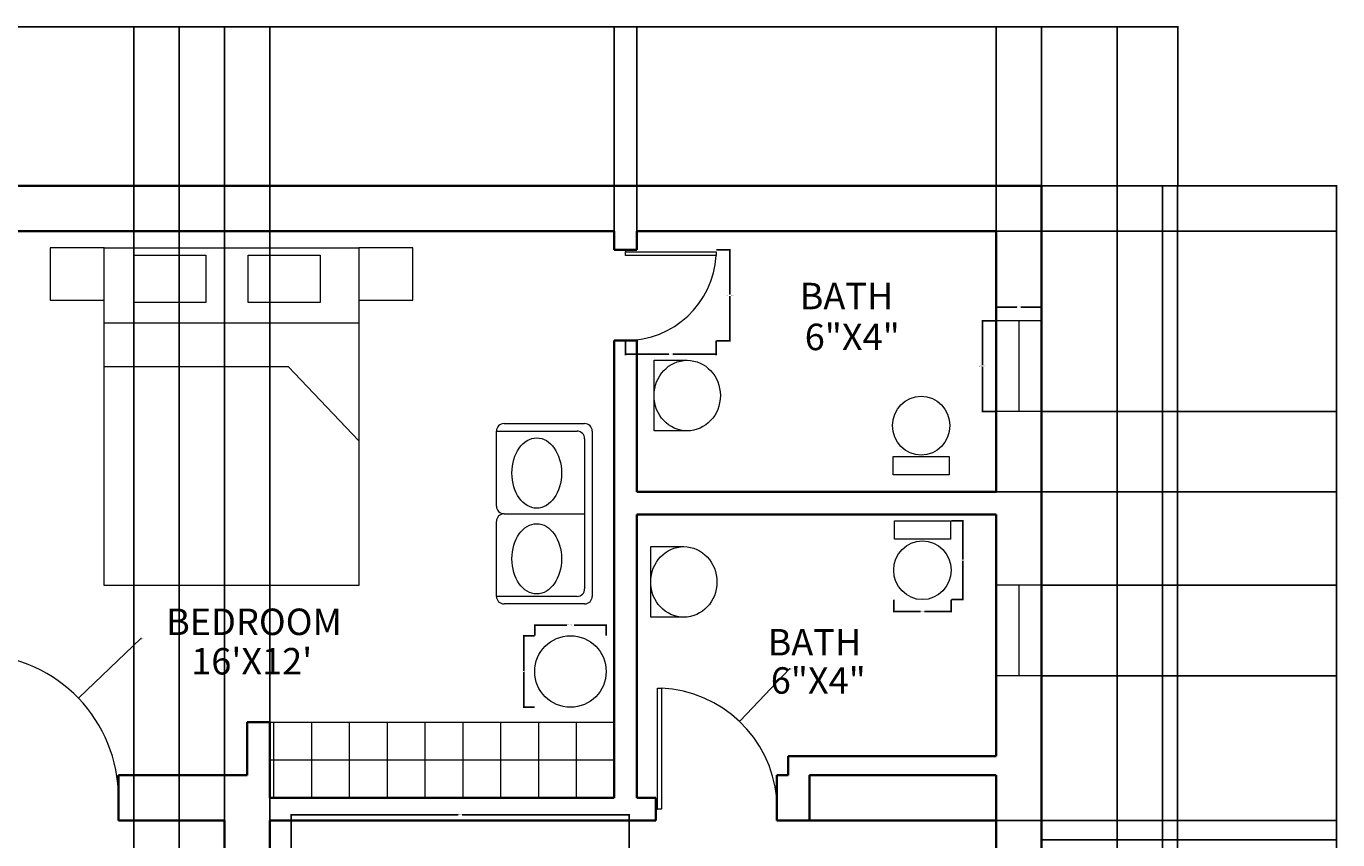
# Model space of a CAD drawing. Units: inches. Extents: x 2863 to 3499, y 1212 to 2136.
# Tile 7 of 7: x 3153 to 3499, y 1921 to 2136. Entities that reach past the tile are written whole.
import ezdxf

# ---------------------------------------------------------------- set-up
doc = ezdxf.new("R2010")
doc.units = ezdxf.units.IN
for name, color, linetype, lineweight in [('A-ANNO-DIMS', 2, 'Continuous', 18), ('A-AREA-IDEN', 7, 'Continuous', 18), ('A-DOOR', 221, 'Continuous', 18), ('A-FLOR-CASE', 254, 'Continuous', 18), ('A-FLOR-FIXT', 254, 'Continuous', 18), ('A-FURN', 131, 'Continuous', 18), ('A-GLAZ', 191, 'Continuous', 18), ('A-WALL', 51, 'Continuous', 35), ('C-PROP', 51, 'Continuous', 25)]:
    doc.layers.add(name, color=color, linetype=linetype, lineweight=lineweight)
doc.styles.get("Standard").update_dxf_attribs({"font": 'arial.ttf'})
doc.dimstyles.get("Standard").update_dxf_attribs({"dimtxt": 0.18, "dimasz": 0.18, "dimexe": 0.18, "dimexo": 0.0625, "dimgap": 0.09, "dimtad": 0, "dimtih": 1, "dimtoh": 1, "dimdec": 4, "dimzin": 0, "dimdsep": 46, "dimtxsty": 'Standard', "dimcen": 0.09, "dimadec": 0, "dimazin": 0, "dimtfac": 1, "dimtdec": 4, "dimtofl": 0, "dimtmove": 0, "dimatfit": 3, "dimfxl": 1, "dimtolj": 1, "dimtzin": 0, "dimarcsym": 0})

# ---------------------------------------------------------------- blocks, each defined once
blk = doc.blocks.new('SOFA-TWO-SEAT')
for p, q in [((0, 45.71), (21.32, 45.71)), ((0, 25.85), (0, 45.71)), ((2, 47.71), (23.32, 47.71)), ((25.32, 45.71), (25.32, 2)), ((23.32, 43.71), (23.32, 4)), ((0, 2), (0, 21.85)), ((2, 23.85), (23.32, 23.85)), ((2, 23.85), (2, 23.85)), ((21.32, 2), (0, 2)), ((23.32, 0), (2, 0))]:
    blk.add_line(p, q)
for centre, start, end in [((2, 45.71), 90, 180), ((21.32, 43.71), 0, 90), ((23.32, 45.71), 0, 90), ((2, 25.85), 180, 270), ((2, 21.85), 90, 180), ((21.32, 4), 270, 0), ((2, 2), 180, 270), ((23.32, 2), 270, 0)]:
    blk.add_arc(centre, 2, start, end)
for centre in [(10.66, 34.63), (10.66, 11.93)]:
    blk.add_ellipse(centre, major_axis=(0, 9.3), ratio=0.704902)
blk = doc.blocks.new('BED-DOUBLE-WITH-NIGHTSTANDS')
for p, q in [((19.89, 14.28), (19.89, 81.52)), ((31.47, 62.91), (51.09, 81.52)), ((31.47, 14.28), (31.47, 62.91))]:
    blk.add_line(p, q)
for points in [[(0, 81.52), (13.89, 81.52), (13.89, 95.8), (0, 95.8)], [(0, 81.52), (89.37, 81.52), (89.37, 14.28), (0, 14.28)], [(2, 71.31), (14.52, 71.31), (14.52, 52.28), (2, 52.28)], [(2, 41.11), (14.52, 41.11), (14.52, 22.08), (2, 22.08)], [(0, 0), (13.89, 0), (13.89, 14.28), (0, 14.28)]]:
    blk.add_lwpolyline(points, close=True)
blk = doc.blocks.new('WC-CLOSE-COUPLED')
blk.add_lwpolyline([(0.19, 20.82), (15, 20.82), (15, 15.96), (0.19, 15.96)], close=True)
blk.add_ellipse((7.6, 7.79), major_axis=(0, 7.78), ratio=0.975839)
blk = doc.blocks.new('TABLE-SIDE-ROUND')
blk.add_circle((9.45, 9.45), 9.45)
blk = doc.blocks.new('BASIN-WALL')
for p, q in [((8.77, 18.68), (17.53, 18.68)), ((17.53, 18.68), (17.53, 0)), ((17.53, 0), (8.77, 0))]:
    blk.add_line(p, q)
blk.add_ellipse((8.77, 9.34), major_axis=(0, 9.34), ratio=0.938307)
blk = doc.blocks.new('DOOR-SWING-24IN')
for p, q in [((0, 0.5), (0, 1.5)), ((0, 1.5), (24, 1.5)), ((24, 0.5), (0, 0.5)), ((24, 1.5), (24, 0.5)), ((24, 0), (24, 0.5))]:
    blk.add_line(p, q)
blk.add_arc((23.95, 0), 24, 89.888, 176.4168)
blk = doc.blocks.new('WINDOW-24IN')
for p, q in [((12, 24), (0, 24)), ((6, 24), (6, 0)), ((12, 0), (0, 0))]:
    blk.add_line(p, q)
blk = doc.blocks.new('*D23')
at = {"layer": 'A-ANNO-DIMS', "color": 0, "lineweight": -2, "transparency": 16777216}
for p, q in [((3397.1, 2005.45), (3400.34, 2005.45)), ((3400.16, 2005.27), (3400.16, 1995.22)), ((3400.16, 1984.81), (3400.16, 1994.86)), ((3397.1, 1984.63), (3400.34, 1984.63))]:
    blk.add_line(p, q, dxfattribs=at)
at = {"layer": 'A-ANNO-DIMS', "color": 0, "transparency": 16777216}
for points in [[(3400.13, 2005.27), (3400.19, 2005.27), (3400.16, 2005.45)], [(3400.13, 1984.81), (3400.19, 1984.81), (3400.16, 1984.63)]]:
    blk.add_solid(points, dxfattribs=at)
at = {"layer": 'Defpoints', "color": 0, "transparency": 16777216}
for p in [(3397.04, 2005.45), (3400.16, 2005.45), (3397.04, 1984.63)]:
    blk.add_point(p, dxfattribs=at)
at = {"layer": 'A-ANNO-DIMS', "color": 0, "transparency": 16777216, "insert": (3400.16, 1995.04), "char_height": 0.18, "attachment_point": 5}
blk.add_mtext('\\A1;WC 21 TYP.', dxfattribs=at)
blk = doc.blocks.new('*D24')
at = {"layer": 'A-ANNO-DIMS', "color": 0, "lineweight": -2, "transparency": 16777216}
for p, q in [((3381.84, 1984.56), (3381.84, 1981.32)), ((3397.04, 1984.56), (3397.04, 1981.32)), ((3382.02, 1981.5), (3388.92, 1981.5)), ((3396.86, 1981.5), (3389.96, 1981.5))]:
    blk.add_line(p, q, dxfattribs=at)
at = {"layer": 'A-ANNO-DIMS', "color": 0, "transparency": 16777216}
for points in [[(3382.02, 1981.53), (3382.02, 1981.47), (3381.84, 1981.5)], [(3396.86, 1981.53), (3396.86, 1981.47), (3397.04, 1981.5)]]:
    blk.add_solid(points, dxfattribs=at)
at = {"layer": 'Defpoints', "color": 0, "transparency": 16777216}
for p in [(3381.84, 1984.63), (3397.04, 1984.63), (3397.04, 1981.5)]:
    blk.add_point(p, dxfattribs=at)
at = {"layer": 'A-ANNO-DIMS', "color": 0, "transparency": 16777216, "insert": (3389.44, 1981.5), "char_height": 0.18, "attachment_point": 5}
blk.add_mtext('\\A1;15 TYP.', dxfattribs=at)
blk = doc.blocks.new('*D25')
at = {"layer": 'A-ANNO-DIMS', "color": 0, "lineweight": -2, "transparency": 16777216}
for p, q in [((3286.93, 1975.12), (3286.93, 1978.07)), ((3287.11, 1977.89), (3295.41, 1977.89)), ((3305.65, 1977.89), (3297.34, 1977.89)), ((3305.83, 1975.12), (3305.83, 1978.07))]:
    blk.add_line(p, q, dxfattribs=at)
at = {"layer": 'A-ANNO-DIMS', "color": 0, "transparency": 16777216}
for points in [[(3287.11, 1977.92), (3287.11, 1977.86), (3286.93, 1977.89)], [(3305.65, 1977.92), (3305.65, 1977.86), (3305.83, 1977.89)]]:
    blk.add_solid(points, dxfattribs=at)
at = {"layer": 'Defpoints', "color": 0, "transparency": 16777216}
for p in [(3305.83, 1977.89), (3286.93, 1975.05), (3305.83, 1975.05)]:
    blk.add_point(p, dxfattribs=at)
at = {"layer": 'A-ANNO-DIMS', "color": 0, "transparency": 16777216, "insert": (3296.38, 1977.89), "char_height": 0.18, "attachment_point": 5}
blk.add_mtext('\\A1;TABLE 19 TYP.', dxfattribs=at)
blk = doc.blocks.new('*D26')
at = {"layer": 'A-ANNO-DIMS', "color": 0, "lineweight": -2, "transparency": 16777216}
for p, q in [((3286.87, 1975.05), (3283.91, 1975.05)), ((3284.09, 1974.87), (3284.09, 1965.79)), ((3284.09, 1956.34), (3284.09, 1965.42)), ((3286.87, 1956.16), (3283.91, 1956.16))]:
    blk.add_line(p, q, dxfattribs=at)
at = {"layer": 'A-ANNO-DIMS', "color": 0, "transparency": 16777216}
for points in [[(3284.06, 1974.87), (3284.12, 1974.87), (3284.09, 1975.05)], [(3284.06, 1956.34), (3284.12, 1956.34), (3284.09, 1956.16)]]:
    blk.add_solid(points, dxfattribs=at)
at = {"layer": 'Defpoints', "color": 0, "transparency": 16777216}
for p in [(3284.09, 1975.05), (3286.93, 1975.05), (3286.93, 1956.16)]:
    blk.add_point(p, dxfattribs=at)
at = {"layer": 'A-ANNO-DIMS', "color": 0, "transparency": 16777216, "insert": (3284.09, 1965.6), "char_height": 0.18, "attachment_point": 5}
blk.add_mtext('\\A1;19 TYP.', dxfattribs=at)
blk = doc.blocks.new('*D31')
at = {"layer": 'A-ANNO-DIMS', "color": 0, "lineweight": -2, "transparency": 16777216}
for p, q in [((3408.85, 2058.44), (3405.14, 2058.44)), ((3405.32, 2058.26), (3405.32, 2046.63)), ((3405.32, 2034.62), (3405.32, 2046.26)), ((3408.85, 2034.44), (3405.14, 2034.44))]:
    blk.add_line(p, q, dxfattribs=at)
at = {"layer": 'A-ANNO-DIMS', "color": 0, "transparency": 16777216}
for points in [[(3405.29, 2058.26), (3405.35, 2058.26), (3405.32, 2058.44)], [(3405.29, 2034.62), (3405.35, 2034.62), (3405.32, 2034.44)]]:
    blk.add_solid(points, dxfattribs=at)
at = {"layer": 'Defpoints', "color": 0, "transparency": 16777216}
for p in [(3405.32, 2058.44), (3408.92, 2058.44), (3408.92, 2034.44)]:
    blk.add_point(p, dxfattribs=at)
at = {"layer": 'A-ANNO-DIMS', "color": 0, "transparency": 16777216, "insert": (3405.32, 2046.44), "char_height": 0.18, "attachment_point": 5}
blk.add_mtext('\\A1;WINDOW 24 TYP.', dxfattribs=at)
blk = doc.blocks.new('*D32')
at = {"layer": 'A-ANNO-DIMS', "color": 0, "lineweight": -2, "transparency": 16777216}
for p, q in [((3408.92, 2058.51), (3408.92, 2062.22)), ((3409.1, 2062.04), (3414.4, 2062.04)), ((3420.74, 2062.04), (3415.44, 2062.04)), ((3420.92, 2058.51), (3420.92, 2062.22))]:
    blk.add_line(p, q, dxfattribs=at)
at = {"layer": 'A-ANNO-DIMS', "color": 0, "transparency": 16777216}
for points in [[(3409.1, 2062.07), (3409.1, 2062.01), (3408.92, 2062.04)], [(3420.74, 2062.07), (3420.74, 2062.01), (3420.92, 2062.04)]]:
    blk.add_solid(points, dxfattribs=at)
at = {"layer": 'Defpoints', "color": 0, "transparency": 16777216}
for p in [(3420.92, 2062.04), (3408.92, 2058.44), (3420.92, 2058.44)]:
    blk.add_point(p, dxfattribs=at)
at = {"layer": 'A-ANNO-DIMS', "color": 0, "transparency": 16777216, "insert": (3414.92, 2062.04), "char_height": 0.18, "attachment_point": 5}
blk.add_mtext('\\A1;12 TYP.', dxfattribs=at)
blk = doc.blocks.new('*D36')
at = {"layer": 'A-ANNO-DIMS', "color": 0, "lineweight": -2, "transparency": 16777216}
for p, q in [((3222.54, 1913.39), (3222.54, 1927.87)), ((3311.9, 1913.39), (3311.9, 1927.87)), ((3222.72, 1927.69), (3266.69, 1927.69)), ((3311.72, 1927.69), (3267.75, 1927.69))]:
    blk.add_line(p, q, dxfattribs=at)
at = {"layer": 'A-ANNO-DIMS', "color": 0, "transparency": 16777216}
for points in [[(3222.72, 1927.72), (3222.72, 1927.66), (3222.54, 1927.69)], [(3311.72, 1927.72), (3311.72, 1927.66), (3311.9, 1927.69)]]:
    blk.add_solid(points, dxfattribs=at)
at = {"layer": 'Defpoints', "color": 0, "transparency": 16777216}
for p in [(3311.9, 1927.69), (3222.54, 1913.32), (3311.9, 1913.32)]:
    blk.add_point(p, dxfattribs=at)
at = {"layer": 'A-ANNO-DIMS', "color": 0, "transparency": 16777216, "insert": (3267.22, 1927.69), "char_height": 0.18, "attachment_point": 5}
blk.add_mtext('\\A1;89 TYP.', dxfattribs=at)
blk = doc.blocks.new('*D43')
at = {"layer": 'A-ANNO-DIMS', "color": 0, "lineweight": -2, "transparency": 16777216}
for p, q in [((3334.98, 2077.17), (3338.7, 2077.17)), ((3338.52, 2076.99), (3338.52, 2065.34)), ((3338.52, 2053.32), (3338.52, 2064.97)), ((3334.98, 2053.14), (3338.7, 2053.14))]:
    blk.add_line(p, q, dxfattribs=at)
at = {"layer": 'A-ANNO-DIMS', "color": 0, "transparency": 16777216}
for points in [[(3338.49, 2076.99), (3338.55, 2076.99), (3338.52, 2077.17)], [(3338.49, 2053.32), (3338.55, 2053.32), (3338.52, 2053.14)]]:
    blk.add_solid(points, dxfattribs=at)
at = {"layer": 'Defpoints', "color": 0, "transparency": 16777216}
for p in [(3334.92, 2077.17), (3334.92, 2053.14), (3338.52, 2053.14)]:
    blk.add_point(p, dxfattribs=at)
at = {"layer": 'A-ANNO-DIMS', "color": 0, "transparency": 16777216, "insert": (3338.52, 2065.15), "char_height": 0.18, "attachment_point": 5}
blk.add_mtext('\\A1;BATH DOOR 24 TYP.', dxfattribs=at)
blk = doc.blocks.new('*D44')
at = {"layer": 'A-ANNO-DIMS', "color": 0, "lineweight": -2, "transparency": 16777216}
for p, q in [((3310.92, 2053.08), (3310.92, 2049.36)), ((3334.92, 2053.08), (3334.92, 2049.36)), ((3311.1, 2049.54), (3322.39, 2049.54)), ((3334.74, 2049.54), (3323.45, 2049.54))]:
    blk.add_line(p, q, dxfattribs=at)
at = {"layer": 'A-ANNO-DIMS', "color": 0, "transparency": 16777216}
for points in [[(3311.1, 2049.57), (3311.1, 2049.51), (3310.92, 2049.54)], [(3334.74, 2049.57), (3334.74, 2049.51), (3334.92, 2049.54)]]:
    blk.add_solid(points, dxfattribs=at)
at = {"layer": 'Defpoints', "color": 0, "transparency": 16777216}
for p in [(3310.92, 2053.14), (3334.92, 2053.14), (3310.92, 2049.54)]:
    blk.add_point(p, dxfattribs=at)
at = {"layer": 'A-ANNO-DIMS', "color": 0, "transparency": 16777216, "insert": (3322.92, 2049.54), "char_height": 0.18, "attachment_point": 5}
blk.add_mtext('\\A1;24 TYP.', dxfattribs=at)
blk = doc.blocks.new('*D52')
at = {"layer": 'A-ANNO-DIMS', "color": 0, "lineweight": -2, "transparency": 16777216}
for p, q in [((2940.92, 2094.23), (2940.92, 2136.37)), ((2941.1, 2136.19), (3180.62, 2136.19)), ((3420.74, 2136.19), (3181.21, 2136.19)), ((3420.92, 2094.23), (3420.92, 2136.37))]:
    blk.add_line(p, q, dxfattribs=at)
at = {"layer": 'A-ANNO-DIMS', "color": 0, "transparency": 16777216}
for points in [[(2941.1, 2136.22), (2941.1, 2136.16), (2940.92, 2136.19)], [(3420.74, 2136.22), (3420.74, 2136.16), (3420.92, 2136.19)]]:
    blk.add_solid(points, dxfattribs=at)
at = {"layer": 'Defpoints', "color": 0, "transparency": 16777216}
for p in [(3420.92, 2136.19), (2940.92, 2094.17), (3420.92, 2094.17)]:
    blk.add_point(p, dxfattribs=at)
at = {"layer": 'A-ANNO-DIMS', "color": 0, "transparency": 16777216, "insert": (3180.92, 2136.19), "char_height": 0.18, "attachment_point": 5}
blk.add_mtext('\\A1;480', dxfattribs=at)
blk = doc.blocks.new('*D53')
at = {"layer": 'A-ANNO-DIMS', "color": 0, "lineweight": -2, "transparency": 16777216}
for p, q in [((3420.92, 2094.23), (3420.92, 2136.37)), ((3421.1, 2136.19), (3438.7, 2136.19)), ((3456.74, 2136.19), (3439.14, 2136.19)), ((3456.92, 2094.23), (3456.92, 2136.37))]:
    blk.add_line(p, q, dxfattribs=at)
at = {"layer": 'A-ANNO-DIMS', "color": 0, "transparency": 16777216}
for points in [[(3421.1, 2136.22), (3421.1, 2136.16), (3420.92, 2136.19)], [(3456.74, 2136.22), (3456.74, 2136.16), (3456.92, 2136.19)]]:
    blk.add_solid(points, dxfattribs=at)
at = {"layer": 'Defpoints', "color": 0, "transparency": 16777216}
for p in [(3456.92, 2136.19), (3420.92, 2094.17), (3456.92, 2094.17)]:
    blk.add_point(p, dxfattribs=at)
at = {"layer": 'A-ANNO-DIMS', "color": 0, "transparency": 16777216, "insert": (3438.92, 2136.19), "char_height": 0.18, "attachment_point": 5}
blk.add_mtext('\\A1;36', dxfattribs=at)
blk = doc.blocks.new('*D55')
at = {"layer": 'A-ANNO-DIMS', "color": 0, "lineweight": -2, "transparency": 16777216}
for p, q in [((3115.92, 2082.23), (3115.92, 2136.37)), ((3116.1, 2136.19), (3211.64, 2136.19)), ((3307.74, 2136.19), (3212.2, 2136.19)), ((3307.92, 2082.23), (3307.92, 2136.37))]:
    blk.add_line(p, q, dxfattribs=at)
at = {"layer": 'A-ANNO-DIMS', "color": 0, "transparency": 16777216}
for points in [[(3116.1, 2136.22), (3116.1, 2136.16), (3115.92, 2136.19)], [(3307.74, 2136.22), (3307.74, 2136.16), (3307.92, 2136.19)]]:
    blk.add_solid(points, dxfattribs=at)
at = {"layer": 'Defpoints', "color": 0, "transparency": 16777216}
for p in [(3307.92, 2136.19), (3115.92, 2082.17), (3307.92, 2082.17)]:
    blk.add_point(p, dxfattribs=at)
at = {"layer": 'A-ANNO-DIMS', "color": 0, "transparency": 16777216, "insert": (3211.92, 2136.19), "char_height": 0.18, "attachment_point": 5}
blk.add_mtext('\\A1;192', dxfattribs=at)
blk = doc.blocks.new('*D56')
at = {"layer": 'A-ANNO-DIMS', "color": 0, "lineweight": -2, "transparency": 16777216}
for p, q in [((3313.92, 2082.23), (3313.92, 2136.37)), ((3314.1, 2136.19), (3361.2, 2136.19)), ((3408.74, 2136.19), (3361.64, 2136.19)), ((3408.92, 2082.23), (3408.92, 2136.37))]:
    blk.add_line(p, q, dxfattribs=at)
at = {"layer": 'A-ANNO-DIMS', "color": 0, "transparency": 16777216}
for points in [[(3314.1, 2136.22), (3314.1, 2136.16), (3313.92, 2136.19)], [(3408.74, 2136.22), (3408.74, 2136.16), (3408.92, 2136.19)]]:
    blk.add_solid(points, dxfattribs=at)
at = {"layer": 'Defpoints', "color": 0, "transparency": 16777216}
for p in [(3408.92, 2136.19), (3313.92, 2082.17), (3408.92, 2082.17)]:
    blk.add_point(p, dxfattribs=at)
at = {"layer": 'A-ANNO-DIMS', "color": 0, "transparency": 16777216, "insert": (3361.42, 2136.19), "char_height": 0.18, "attachment_point": 5}
blk.add_mtext('\\A1;95', dxfattribs=at)
blk = doc.blocks.new('*D57')
at = {"layer": 'A-ANNO-DIMS', "color": 0, "lineweight": -2, "transparency": 16777216}
for p, q in [((3456.98, 2094.17), (3499.12, 2094.17)), ((3498.94, 2093.99), (3498.94, 1734.35)), ((3498.94, 1374.35), (3498.94, 1733.98)), ((3452.98, 1374.17), (3499.12, 1374.17))]:
    blk.add_line(p, q, dxfattribs=at)
at = {"layer": 'A-ANNO-DIMS', "color": 0, "transparency": 16777216}
for points in [[(3498.91, 2093.99), (3498.97, 2093.99), (3498.94, 2094.17)], [(3498.91, 1374.35), (3498.97, 1374.35), (3498.94, 1374.17)]]:
    blk.add_solid(points, dxfattribs=at)
at = {"layer": 'Defpoints', "color": 0, "transparency": 16777216}
for p in [(3456.92, 2094.17), (3498.94, 2094.17), (3452.92, 1374.17)]:
    blk.add_point(p, dxfattribs=at)
at = {"layer": 'A-ANNO-DIMS', "color": 0, "transparency": 16777216, "insert": (3498.94, 1734.17), "char_height": 0.18, "attachment_point": 5}
blk.add_mtext('\\A1;720', dxfattribs=at)
blk = doc.blocks.new('*D61')
at = {"layer": 'A-ANNO-DIMS', "color": 0, "lineweight": -2, "transparency": 16777216}
for p, q in [((3408.98, 1926.17), (3499.12, 1926.17)), ((3498.94, 1925.99), (3498.94, 1836.35)), ((3498.94, 1746.35), (3498.94, 1835.98)), ((3408.98, 1746.17), (3499.12, 1746.17))]:
    blk.add_line(p, q, dxfattribs=at)
at = {"layer": 'A-ANNO-DIMS', "color": 0, "transparency": 16777216}
for points in [[(3498.91, 1925.99), (3498.97, 1925.99), (3498.94, 1926.17)], [(3498.91, 1746.35), (3498.97, 1746.35), (3498.94, 1746.17)]]:
    blk.add_solid(points, dxfattribs=at)
at = {"layer": 'Defpoints', "color": 0, "transparency": 16777216}
for p in [(3408.92, 1926.17), (3498.94, 1926.17), (3408.92, 1746.17)]:
    blk.add_point(p, dxfattribs=at)
at = {"layer": 'A-ANNO-DIMS', "color": 0, "transparency": 16777216, "insert": (3498.94, 1836.17), "char_height": 0.18, "attachment_point": 5}
blk.add_mtext('\\A1;180', dxfattribs=at)
blk = doc.blocks.new('*D62')
at = {"layer": 'A-ANNO-DIMS', "color": 0, "lineweight": -2, "transparency": 16777216}
for p, q in [((3408.98, 2013.17), (3499.12, 2013.17)), ((3498.94, 2012.99), (3498.94, 1969.85)), ((3498.94, 1926.35), (3498.94, 1969.48)), ((3408.98, 1926.17), (3499.12, 1926.17))]:
    blk.add_line(p, q, dxfattribs=at)
at = {"layer": 'A-ANNO-DIMS', "color": 0, "transparency": 16777216}
for points in [[(3498.91, 2012.99), (3498.97, 2012.99), (3498.94, 2013.17)], [(3498.91, 1926.35), (3498.97, 1926.35), (3498.94, 1926.17)]]:
    blk.add_solid(points, dxfattribs=at)
at = {"layer": 'Defpoints', "color": 0, "transparency": 16777216}
for p in [(3408.92, 2013.17), (3498.94, 2013.17), (3408.92, 1926.17)]:
    blk.add_point(p, dxfattribs=at)
at = {"layer": 'A-ANNO-DIMS', "color": 0, "transparency": 16777216, "insert": (3498.94, 1969.67), "char_height": 0.18, "attachment_point": 5}
blk.add_mtext('\\A1;87', dxfattribs=at)
blk = doc.blocks.new('*D63')
at = {"layer": 'A-ANNO-DIMS', "color": 0, "lineweight": -2, "transparency": 16777216}
for p, q in [((3408.98, 2082.17), (3499.12, 2082.17)), ((3498.94, 2081.99), (3498.94, 2047.85)), ((3498.94, 2013.35), (3498.94, 2047.48)), ((3408.98, 2013.17), (3499.12, 2013.17))]:
    blk.add_line(p, q, dxfattribs=at)
at = {"layer": 'A-ANNO-DIMS', "color": 0, "transparency": 16777216}
for points in [[(3498.91, 2081.99), (3498.97, 2081.99), (3498.94, 2082.17)], [(3498.91, 2013.35), (3498.97, 2013.35), (3498.94, 2013.17)]]:
    blk.add_solid(points, dxfattribs=at)
at = {"layer": 'Defpoints', "color": 0, "transparency": 16777216}
for p in [(3408.92, 2082.17), (3498.94, 2082.17), (3408.92, 2013.17)]:
    blk.add_point(p, dxfattribs=at)
at = {"layer": 'A-ANNO-DIMS', "color": 0, "transparency": 16777216, "insert": (3498.94, 2047.67), "char_height": 0.18, "attachment_point": 5}
blk.add_mtext('\\A1;69', dxfattribs=at)
blk = doc.blocks.new('*D72')
at = {"layer": 'A-ANNO-DIMS', "color": 0, "lineweight": -2, "transparency": 16777216}
for p, q in [((3133.92, 1549.23), (3133.92, 2136.37)), ((3134.1, 2136.19), (3169.22, 2136.19)), ((3204.74, 2136.19), (3169.62, 2136.19)), ((3204.92, 1561.23), (3204.92, 2136.37))]:
    blk.add_line(p, q, dxfattribs=at)
at = {"layer": 'A-ANNO-DIMS', "color": 0, "transparency": 16777216}
for points in [[(3134.1, 2136.22), (3134.1, 2136.16), (3133.92, 2136.19)], [(3204.74, 2136.22), (3204.74, 2136.16), (3204.92, 2136.19)]]:
    blk.add_solid(points, dxfattribs=at)
at = {"layer": 'Defpoints', "color": 0, "transparency": 16777216}
for p in [(3204.92, 2136.19), (3204.92, 1561.17), (3133.92, 1549.17)]:
    blk.add_point(p, dxfattribs=at)
at = {"layer": 'A-ANNO-DIMS', "color": 0, "transparency": 16777216, "insert": (3169.42, 2136.19), "char_height": 0.18, "attachment_point": 5}
blk.add_mtext('\\A1;71', dxfattribs=at)
blk = doc.blocks.new('*D99')
at = {"layer": 'A-ANNO-DIMS', "color": 0, "lineweight": -2, "transparency": 16777216}
for p, q in [((3420.98, 1964.48), (3499.12, 1964.48)), ((3498.94, 1964.3), (3498.94, 1942.96)), ((3498.94, 1921.26), (3498.94, 1942.6)), ((3420.98, 1921.08), (3499.12, 1921.08))]:
    blk.add_line(p, q, dxfattribs=at)
at = {"layer": 'A-ANNO-DIMS', "color": 0, "transparency": 16777216}
for points in [[(3498.91, 1964.3), (3498.97, 1964.3), (3498.94, 1964.48)], [(3498.91, 1921.26), (3498.97, 1921.26), (3498.94, 1921.08)]]:
    blk.add_solid(points, dxfattribs=at)
at = {"layer": 'Defpoints', "color": 0, "transparency": 16777216}
for p in [(3420.92, 1964.48), (3498.94, 1964.48), (3420.92, 1921.08)]:
    blk.add_point(p, dxfattribs=at)
at = {"layer": 'A-ANNO-DIMS', "color": 0, "transparency": 16777216, "insert": (3498.94, 1942.78), "char_height": 0.18, "attachment_point": 5}
blk.add_mtext('\\A1;43.4', dxfattribs=at)
blk = doc.blocks.new('*D100')
at = {"layer": 'A-ANNO-DIMS', "color": 0, "lineweight": -2, "transparency": 16777216}
for p, q in [((3420.98, 2034.44), (3499.12, 2034.44)), ((3498.94, 2034.26), (3498.94, 2011.64)), ((3498.94, 1988.66), (3498.94, 2011.28)), ((3420.98, 1988.48), (3499.12, 1988.48))]:
    blk.add_line(p, q, dxfattribs=at)
at = {"layer": 'A-ANNO-DIMS', "color": 0, "transparency": 16777216}
for points in [[(3498.91, 2034.26), (3498.97, 2034.26), (3498.94, 2034.44)], [(3498.91, 1988.66), (3498.97, 1988.66), (3498.94, 1988.48)]]:
    blk.add_solid(points, dxfattribs=at)
at = {"layer": 'Defpoints', "color": 0, "transparency": 16777216}
for p in [(3420.92, 2034.44), (3498.94, 2034.44), (3420.92, 1988.48)]:
    blk.add_point(p, dxfattribs=at)
at = {"layer": 'A-ANNO-DIMS', "color": 0, "transparency": 16777216, "insert": (3498.94, 2011.46), "char_height": 0.18, "attachment_point": 5}
blk.add_mtext('\\A1;45.97', dxfattribs=at)
blk = doc.blocks.new('*D107')
at = {"layer": 'A-ANNO-DIMS', "color": 0, "lineweight": -2, "transparency": 16777216}
for p, q in [((3216.92, 1270.23), (3216.92, 2136.37)), ((3217.1, 2136.19), (3328.63, 2136.19)), ((3440.74, 2136.19), (3329.21, 2136.19)), ((3440.92, 1270.23), (3440.92, 2136.37))]:
    blk.add_line(p, q, dxfattribs=at)
at = {"layer": 'A-ANNO-DIMS', "color": 0, "transparency": 16777216}
for points in [[(3217.1, 2136.22), (3217.1, 2136.16), (3216.92, 2136.19)], [(3440.74, 2136.22), (3440.74, 2136.16), (3440.92, 2136.19)]]:
    blk.add_solid(points, dxfattribs=at)
at = {"layer": 'Defpoints', "color": 0, "transparency": 16777216}
for p in [(3440.92, 2136.19), (3216.92, 1270.17), (3440.92, 1270.17)]:
    blk.add_point(p, dxfattribs=at)
at = {"layer": 'A-ANNO-DIMS', "color": 0, "transparency": 16777216, "insert": (3328.92, 2136.19), "char_height": 0.18, "attachment_point": 5}
blk.add_mtext('\\A1;224', dxfattribs=at)
blk = doc.blocks.new('*D110')
at = {"layer": 'A-ANNO-DIMS', "color": 0, "lineweight": -2, "transparency": 16777216}
for p, q in [((3180.92, 1374.23), (3180.92, 2136.37)), ((3181.1, 2136.19), (3186.71, 2136.19)), ((3192.74, 2136.19), (3187.13, 2136.19)), ((3192.92, 1374.23), (3192.92, 2136.37))]:
    blk.add_line(p, q, dxfattribs=at)
at = {"layer": 'A-ANNO-DIMS', "color": 0, "transparency": 16777216}
for points in [[(3181.1, 2136.22), (3181.1, 2136.16), (3180.92, 2136.19)], [(3192.74, 2136.22), (3192.74, 2136.16), (3192.92, 2136.19)]]:
    blk.add_solid(points, dxfattribs=at)
at = {"layer": 'Defpoints', "color": 0, "transparency": 16777216}
for p in [(3192.92, 2136.19), (3180.92, 1374.17), (3192.92, 1374.17)]:
    blk.add_point(p, dxfattribs=at)
at = {"layer": 'A-ANNO-DIMS', "color": 0, "transparency": 16777216, "insert": (3186.92, 2136.19), "char_height": 0.18, "attachment_point": 5}
blk.add_mtext('\\A1;12', dxfattribs=at)
blk = doc.blocks.new('*D114')
at = {"layer": 'A-ANNO-DIMS', "color": 0, "lineweight": -2, "transparency": 16777216}
for p, q in [((3182.77, 1974.31), (3166.45, 1958.64)), ((3182.95, 1974.31), (3182.77, 1974.31)), ((3138.83, 1932.19), (3139.01, 1932.19)), ((3138.92, 1932.1), (3138.92, 1932.28))]:
    blk.add_line(p, q, dxfattribs=at)
at = {"layer": 'A-ANNO-DIMS', "color": 0, "transparency": 16777216}
blk.add_solid([(3166.43, 1958.66), (3166.47, 1958.62), (3166.32, 1958.52)], dxfattribs=at)
at = {"layer": 'Defpoints', "color": 0, "transparency": 16777216}
for p in [(3166.32, 1958.52), (3138.92, 1932.19)]:
    blk.add_point(p, dxfattribs=at)
at = {"layer": 'A-ANNO-DIMS', "color": 0, "transparency": 16777216, "insert": (3183.45, 1974.31), "char_height": 0.18, "attachment_point": 5}
blk.add_mtext('\\A1;2X R38', dxfattribs=at)
blk = doc.blocks.new('*D116')
at = {"layer": 'A-ANNO-DIMS', "color": 0, "lineweight": -2, "transparency": 16777216}
for p, q in [((3354.33, 1966.3), (3341.23, 1952.52)), ((3354.51, 1966.3), (3354.33, 1966.3)), ((3318.96, 1929.19), (3319.14, 1929.19)), ((3319.05, 1929.1), (3319.05, 1929.28))]:
    blk.add_line(p, q, dxfattribs=at)
at = {"layer": 'A-ANNO-DIMS', "color": 0, "transparency": 16777216}
blk.add_solid([(3341.21, 1952.54), (3341.25, 1952.49), (3341.1, 1952.38)], dxfattribs=at)
at = {"layer": 'Defpoints', "color": 0, "transparency": 16777216}
for p in [(3341.1, 1952.38), (3319.05, 1929.19)]:
    blk.add_point(p, dxfattribs=at)
at = {"layer": 'A-ANNO-DIMS', "color": 0, "transparency": 16777216, "insert": (3354.82, 1966.3), "char_height": 0.18, "attachment_point": 5}
blk.add_mtext('\\A1;R32', dxfattribs=at)

msp = doc.modelspace()

# ---------------------------------------------------------------- linework, layer by layer
at = {"layer": 'A-DOOR'}
for p, q in [((3319.4168, 1929.1651), (3319.4168, 1961.1651)), ((3319.4168, 1961.1651), (3320.4168, 1961.1651)), ((3320.4168, 1961.1651), (3320.4168, 1929.1651)), ((3318.9168, 1929.1651), (3319.4168, 1929.1651)), ((3320.4168, 1929.1651), (3319.4168, 1929.1651))]:
    msp.add_line(p, q, dxfattribs=at)
for centre, radius, start, end in [((3138.9168, 1932.1947), 38, 359.955345, 87.737754), ((3319.055, 1929.1941), 32, 5.327247, 87.561004)]:
    msp.add_arc(centre, radius, start, end, dxfattribs=at)
at = {"layer": 'A-FLOR-CASE'}
for p, q in [((3216.9168, 1952.1651), (3307.9168, 1952.1651)), ((3217.9168, 1952.1651), (3217.9168, 1932.1651)), ((3227.9168, 1952.1651), (3227.9168, 1932.1651)), ((3237.9168, 1952.1651), (3237.9168, 1932.1651)), ((3247.9168, 1952.1651), (3247.9168, 1932.1651)), ((3257.9168, 1952.1651), (3257.9168, 1932.1651)), ((3267.9168, 1952.1651), (3267.9168, 1932.1651)), ((3277.9168, 1952.1651), (3277.9168, 1932.1651)), ((3287.9168, 1952.1651), (3287.9168, 1932.1651)), ((3297.9168, 1952.1651), (3297.9168, 1932.1651)), ((3307.9168, 1952.1651), (3307.9168, 1932.1651)), ((3307.9168, 1942.1651), (3216.9168, 1942.1651))]:
    msp.add_line(p, q, dxfattribs=at)
at = {"layer": 'A-WALL'}
for p, q in [((3115.9168, 2082.1651), (3307.9168, 2082.1651)), ((3307.9168, 2082.1651), (3307.9168, 2077.1651)), ((3307.9168, 2077.1651), (3307.9168, 2082.1651)), ((3313.9168, 2082.1651), (3408.9168, 2082.1651)), ((3313.9168, 2077.1651), (3313.9168, 2082.1651)), ((3408.9168, 2082.1651), (3408.9168, 2013.1651)), ((3307.9168, 2077.1651), (3313.9168, 2077.1651)), ((3307.9168, 1938.1651), (3307.9168, 2053.1651)), ((3307.9168, 2053.1651), (3313.9168, 2053.1651)), ((3313.9168, 2013.1651), (3313.9168, 2053.1651)), ((3313.9168, 2013.1651), (3408.9168, 2013.1651)), ((3313.9168, 1938.1651), (3313.9168, 2007.1651)), ((3313.9168, 2007.1651), (3408.9168, 2007.1651)), ((3408.9168, 2007.1651), (3408.9168, 1943.1651)), ((3210.9168, 1938.1651), (3210.9168, 1952.1651)), ((3210.9168, 1952.1651), (3216.9168, 1952.1651)), ((3216.9168, 1952.1651), (3216.9168, 1938.1651)), ((3353.9168, 1938.1651), (3353.9168, 1943.1651)), ((3353.9168, 1943.1651), (3408.9168, 1943.1651)), ((3176.9168, 1926.1651), (3176.9168, 1938.1651)), ((3176.9168, 1938.1651), (3210.9168, 1938.1651)), ((3216.9168, 1938.1651), (3216.9168, 1932.1651)), ((3307.9168, 1932.1651), (3307.9168, 1938.1651)), ((3313.9168, 1938.1651), (3313.9168, 1932.1651)), ((3350.9168, 1938.1651), (3350.9168, 1926.1651)), ((3350.9168, 1938.1651), (3353.9168, 1938.1651)), ((3350.9168, 1938.1651), (3353.9168, 1938.1651)), ((3359.5654, 1938.1651), (3359.5654, 1926.1651)), ((3359.5654, 1938.1651), (3408.9168, 1938.1651)), ((3408.9168, 1938.1651), (3408.9168, 1926.1651)), ((3216.9168, 1932.1651), (3307.9168, 1932.1651)), ((3313.9168, 1932.1651), (3318.9168, 1932.1651)), ((3318.9168, 1932.1651), (3318.9168, 1926.1651)), ((3176.9168, 1926.1651), (3204.9168, 1926.1651)), ((3204.9168, 1926.1651), (3204.9168, 1806.1651)), ((3216.9168, 1926.1651), (3216.9168, 1806.1651)), ((3216.9168, 1926.1651), (3318.9168, 1926.1651)), ((3350.9168, 1926.1651), (3408.9168, 1926.1651)), ((3408.9168, 1926.1651), (3408.9168, 1561.1651))]:
    msp.add_line(p, q, dxfattribs=at)
msp.add_lwpolyline([(2940.9168, 1453.1651), (2940.9168, 2094.1651), (3420.9168, 2094.1651), (3420.9168, 1374.1651), (3216.9168, 1374.1651)], dxfattribs=at)
at = {"layer": 'C-PROP'}
for p, q in [((2904.9168, 2094.1651), (3456.9168, 2094.1651)), ((3456.9168, 2094.1651), (3420.9168, 2094.1651)), ((3452.9168, 1258.1651), (3452.9168, 2094.1651)), ((3456.9168, 2094.1651), (3456.9168, 1254.1651))]:
    msp.add_line(p, q, dxfattribs=at)

# ---------------------------------------------------------------- block references
at = {"layer": 'A-DOOR', "rotation": 180}
msp.add_blockref('DOOR-SWING-24IN', (3334.9165, 2077.1652), dxfattribs=at)
at = {"layer": 'A-FLOR-FIXT', "rotation": 180}
for name, p in [('BASIN-WALL', (3336.0181, 2047.9592)), ('WC-CLOSE-COUPLED', (3396.7096, 2038.4642)), ('BASIN-WALL', (3335.1328, 1998.6473))]:
    msp.add_blockref(name, p, dxfattribs=at)
at = {"layer": 'A-FLOR-FIXT'}
msp.add_blockref('WC-CLOSE-COUPLED', (3381.8439, 1984.6259), dxfattribs=at)
at = {"layer": 'A-FURN', "rotation": 269.9999999999988}
msp.add_blockref('BED-DOUBLE-WITH-NIGHTSTANDS', (3158.8772, 2077.7591), dxfattribs=at)
at = {"layer": 'A-FURN'}
for name, p in [('SOFA-TWO-SEAT', (3276.822, 1983.498)), ('TABLE-SIDE-ROUND', (3286.929, 1956.156))]:
    msp.add_blockref(name, p, dxfattribs=at)
at = {"layer": 'A-GLAZ'}
for p in [(3408.917, 2034.4449), (3408.917, 1964.4771)]:
    msp.add_blockref('WINDOW-24IN', p, dxfattribs=at)

# ---------------------------------------------------------------- texts
at = {"layer": 'A-AREA-IDEN'}
for tag, p in [('BATH', (3356.9751, 2061.4647)), ('6"X4"', (3358.3244, 2050.6453)), ('BEDROOM', (3189.4913, 1975.2591)), ('BATH', (3348.5033, 1969.8481)), ("16'X12'", (3196.136, 1964.8264)), ('6"X4"', (3349.3464, 1959.7363))]:
    msp.add_attdef(tag, p, '', height=7, dxfattribs=at)

# ---------------------------------------------------------------- dimensions: what is measured, and where the dimension line sits
at = {"layer": 'A-ANNO-DIMS'}
for base, p1, p2, picture, middle in [((3420.9168, 2136.1851), (2940.9168, 2094.1651), (3420.9168, 2094.1651), '*D52', (3180.9168, 2136.1851)), ((3307.9168, 2136.1851), (3115.9168, 2082.1651), (3307.9168, 2082.1651), '*D55', (3211.9168, 2136.1851)), ((3204.9168, 2136.1851), (3133.9168, 1549.1651), (3204.9168, 1561.1651), '*D72', (3169.4168, 2136.1851)), ((3192.9168, 2136.1851), (3180.9168, 1374.1651), (3192.9168, 1374.1651), '*D110', (3186.9168, 2136.1851)), ((3440.9168, 2136.1851), (3216.9168, 1270.1651), (3440.9168, 1270.1651), '*D107', (3328.9168, 2136.1851)), ((3408.9168, 2136.1851), (3313.9168, 2082.1651), (3408.9168, 2082.1651), '*D56', (3361.4168, 2136.1851)), ((3456.9168, 2136.1851), (3420.9168, 2094.1651), (3456.9168, 2094.1651), '*D53', (3438.9168, 2136.1851))]:
    dim = msp.add_linear_dim(base=base, p1=p1, p2=p2, dimstyle='Standard', override={"dimdec": 0, "dimlfac": 1, "dimrnd": 0, "dimzin": 0, "dimdsep": 46, "dimlunit": 2}, dxfattribs=at)
    dim.commit()
    dim.dimension.update_dxf_attribs({"geometry": picture, "text_midpoint": middle})
for base, p1, p2, override, picture, middle in [((3498.9368, 2094.1651), (3452.9168, 1374.1651), (3456.9168, 2094.1651), {"dimdec": 0, "dimlfac": 1, "dimrnd": 0, "dimzin": 0, "dimdsep": 46, "dimlunit": 2}, '*D57', (3498.9368, 1734.1651)), ((3498.9368, 2082.1651), (3408.9168, 2013.1651), (3408.9168, 2082.1651), {"dimdec": 0, "dimlfac": 1, "dimrnd": 0, "dimzin": 0, "dimdsep": 46, "dimlunit": 2}, '*D63', (3498.9368, 2047.6651)), ((3498.9368, 2034.4444), (3420.9168, 1988.4767), (3420.9168, 2034.4444), {"dimdec": 2, "dimlfac": 1, "dimrnd": 0, "dimzin": 0, "dimdsep": 46, "dimlunit": 2}, '*D100', (3498.9368, 2011.4605)), ((3498.9368, 2013.1651), (3408.9168, 1926.1651), (3408.9168, 2013.1651), {"dimdec": 0, "dimlfac": 1, "dimrnd": 0, "dimzin": 0, "dimdsep": 46, "dimlunit": 2}, '*D62', (3498.9368, 1969.6651)), ((3498.9368, 1964.4767), (3420.9168, 1921.0807), (3420.9168, 1964.4767), {"dimdec": 1, "dimlfac": 1, "dimrnd": 0, "dimzin": 0, "dimdsep": 46, "dimlunit": 2}, '*D99', (3498.9368, 1942.7787)), ((3498.9368, 1926.1651), (3408.9168, 1746.1651), (3408.9168, 1926.1651), {"dimdec": 0, "dimlfac": 1, "dimrnd": 0, "dimzin": 0, "dimdsep": 46, "dimlunit": 2}, '*D61', (3498.9368, 1836.1651))]:
    dim = msp.add_linear_dim(base=base, p1=p1, p2=p2, angle=90, dimstyle='Standard', override=override, dxfattribs=at)
    dim.commit()
    dim.dimension.update_dxf_attribs({"geometry": picture, "text_midpoint": middle})
for base, p1, p2, angle, text, picture, middle in [((3338.5205, 2053.1403), (3334.9168, 2077.1651), (3334.9168, 2053.1403), 270, 'BATH DOOR <> TYP.', '*D43', (3338.5205, 2065.1527)), ((3405.3168, 2058.4444), (3408.9168, 2034.4444), (3408.9168, 2058.4444), 90, 'WINDOW <> TYP.', '*D31', (3405.3168, 2046.4444)), ((3310.9168, 2049.5366), (3334.9168, 2053.1403), (3310.9168, 2053.1403), 180, '<> TYP.', '*D44', (3322.9168, 2049.5366)), ((3400.161, 2005.4508), (3397.0373, 1984.6261), (3397.0373, 2005.4508), 90, 'WC <> TYP.', '*D23', (3400.161, 1995.0384)), ((3284.094, 1975.0531), (3286.9285, 1956.1563), (3286.9285, 1975.0531), 90, '<> TYP.', '*D26', (3284.094, 1965.6047))]:
    dim = msp.add_linear_dim(base=base, p1=p1, p2=p2, angle=angle, text=text, dimstyle='Standard', override={"dimdec": 0, "dimlfac": 1, "dimrnd": 0, "dimzin": 0, "dimdsep": 46, "dimlunit": 2}, dxfattribs=at)
    dim.commit()
    dim.dimension.update_dxf_attribs({"geometry": picture, "text_midpoint": middle})
for base, p1, p2, text, picture, middle in [((3420.9168, 2062.0444), (3408.9168, 2058.4444), (3420.9168, 2058.4444), '<> TYP.', '*D32', (3414.9168, 2062.0444)), ((3397.0373, 1981.5024), (3381.8436, 1984.6261), (3397.0373, 1984.6261), '<> TYP.', '*D24', (3389.4405, 1981.5024)), ((3305.8253, 1977.8876), (3286.9285, 1975.0531), (3305.8253, 1975.0531), 'TABLE <> TYP.', '*D25', (3296.3769, 1977.8876)), ((3311.9025, 1927.6929), (3222.5365, 1913.3235), (3311.9025, 1913.3235), '<> TYP.', '*D36', (3267.2195, 1927.6929))]:
    dim = msp.add_linear_dim(base=base, p1=p1, p2=p2, text=text, dimstyle='Standard', override={"dimdec": 0, "dimlfac": 1, "dimrnd": 0, "dimzin": 0, "dimdsep": 46, "dimlunit": 2}, dxfattribs=at)
    dim.commit()
    dim.dimension.update_dxf_attribs({"geometry": picture, "text_midpoint": middle})
dim = msp.add_radius_dim(center=(3138.9168, 1932.1947), mpoint=(3166.3224, 1958.5183), text='2X <>', dimstyle='Standard', override={"dimdec": 0, "dimlfac": 1, "dimrnd": 0, "dimzin": 0, "dimdsep": 46, "dimlunit": 2}, dxfattribs=at)
dim.commit()
dim.dimension.update_dxf_attribs({"geometry": '*D114', "text_midpoint": (3183.4459, 1974.3125), "dimtype": 164})
dim = msp.add_radius_dim(center=(3319.055, 1929.1941), mpoint=(3341.1048, 1952.3847), dimstyle='Standard', override={"dimdec": 0, "dimlfac": 1, "dimrnd": 0, "dimzin": 0, "dimdsep": 46, "dimlunit": 2}, dxfattribs=at)
dim.commit()
dim.dimension.update_dxf_attribs({"geometry": '*D116', "text_midpoint": (3354.8188, 1966.2991), "dimtype": 164})

doc.saveas('drawing.dxf')
